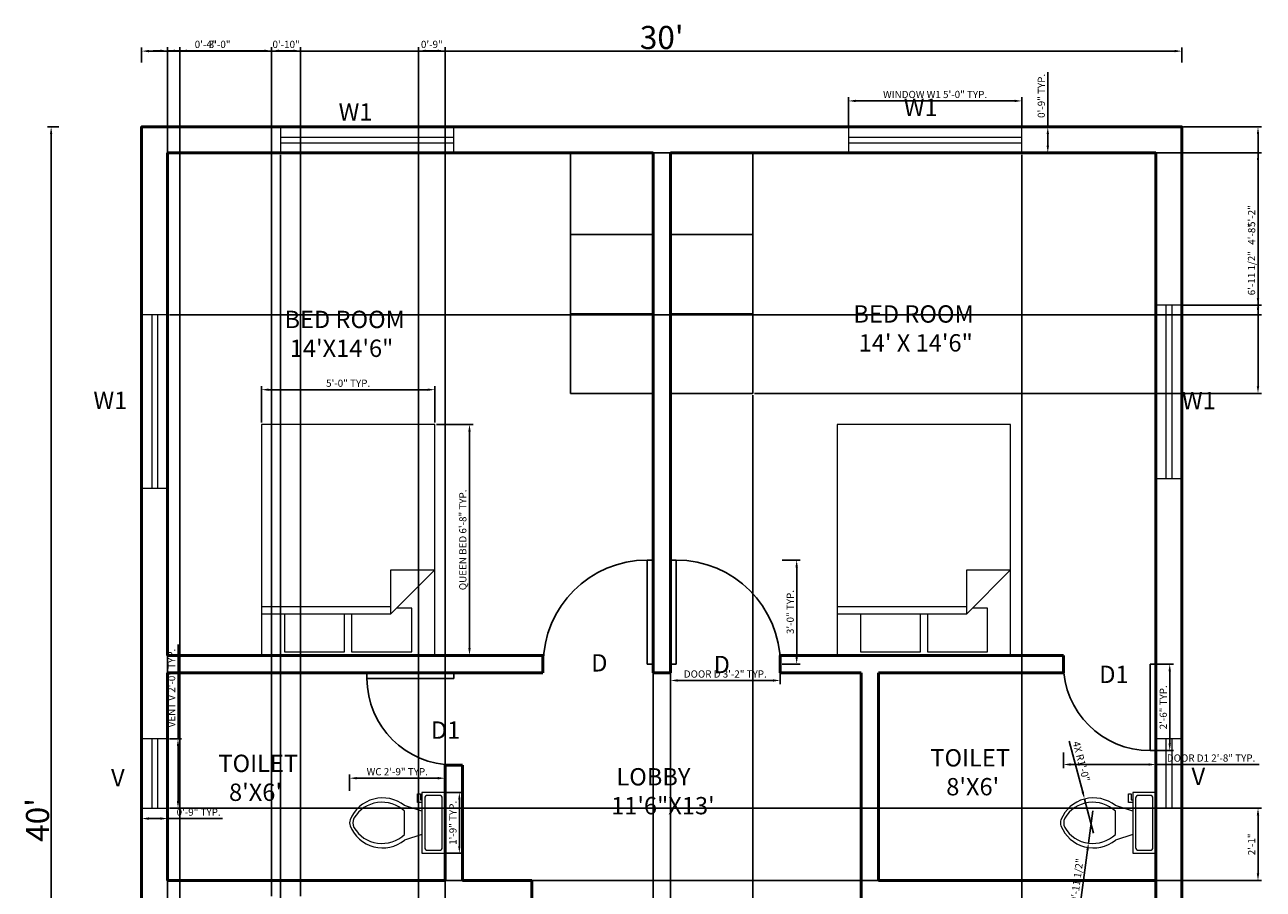
# Model space of a CAD drawing. Units: inches. Extents: x 2936 to 3364, y 2324 to 2867.
# Tile 4 of 4: x 2936 to 3364, y 2568 to 2867. Entities that reach past the tile are written whole.
import ezdxf

# ---------------------------------------------------------------- set-up
doc = ezdxf.new("R2010")
doc.units = ezdxf.units.IN
for name, color, linetype, lineweight in [('A-ANNO-DIMS', 2, 'Continuous', 18), ('A-ANNO-TEXT', 7, 'Continuous', 18), ('A-AREA-IDEN', 7, 'Continuous', 25), ('A-DOOR', 3, 'Continuous', 25), ('A-FLOR-CASE', 9, 'Continuous', 25), ('A-FLOR-FIXT', 9, 'Continuous', 18), ('A-FURN', 8, 'Continuous', 18), ('A-GLAZ', 4, 'Continuous', 18), ('A-WALL', 7, 'Continuous', 50)]:
    doc.layers.add(name, color=color, linetype=linetype, lineweight=lineweight)
doc.styles.get("Standard").update_dxf_attribs({"font": 'arial.ttf'})
doc.dimstyles.new('ISO-25', dxfattribs={"dimtxt": 2.5, "dimasz": 2.5, "dimexe": 1.25, "dimexo": 0.625, "dimtad": 1, "dimdec": 0, "dimlunit": 4, "dimtxsty": 'Standard', "dimcen": 2.5, "dimadec": 0, "dimazin": 0, "dimtfac": 1, "dimtdec": 0, "dimtmove": 0, "dimatfit": 3, "dimfxl": 1, "dimarcsym": 0})

# ---------------------------------------------------------------- blocks, each defined once
blk = doc.blocks.new('Toilet - top')
for p, q in [((9.5, -6), (9.5, -2)), ((-10, -8.5), (-8, -8.5)), ((-10, -9.5), (-10, -8.5)), ((-8, -8.5), (-8, -8)), ((-7, -8), (-7, -9.5)), ((-4, -8), (-6, -14)), ((4, -8), (6, -14)), ((-7, -9.5), (-10, -9.5)), ((4, -14), (-4, -14))]:
    blk.add_line(p, q)
blk.add_lwpolyline([(10.5, -8), (10.5, 0), (-10.5, 0), (-10.5, -8)], close=True)
for points in [[(-9.5, -2), (-9.5, -6)], [(8.5, -1), (-8.5, -1)], [(-8.5, -7), (8.5, -7)]]:
    blk.add_lwpolyline(points)
for centre, radius, start, end in [((-8.62, -1.88), 0.884, 81.8699, 188.1301), ((8.62, -1.88), 0.884, 351.8699, 98.1301), ((-8.62, -6.12), 0.884, 171.8699, 278.1301), ((8.62, -6.12), 0.884, 261.8699, 8.1301), ((3.52, -21.58), 12.17, 141.4691, 247.9714), ((4.2, -21.82), 11.33, 136.3677, 238.9468), ((-3.52, -21.58), 12.17, 292.0284, 38.5307), ((-4.2, -21.82), 11.33, 301.053, 43.6321), ((0, -27.88), 4, 245.7318, 294.2682), ((0, -29), 4, 254.8605, 285.1395)]:
    blk.add_arc(centre, radius, start, end)
blk = doc.blocks.new('Bed - Queen')
for p, q in [((0, -80.00003), (0, 0)), ((0, 0), (59.99999, 0)), ((59.99999, 0), (59.99999, -80.00003)), ((7.99999, -1.2), (28.79998, -1.2)), ((7.99999, -14.4), (7.99999, -1.2)), ((28.79998, -1.2), (28.79998, -14.4)), ((31.19999, -1.2), (51.99999, -1.2)), ((31.19999, -14.4), (31.19999, -1.2)), ((51.99999, -1.2), (51.99999, -16.4)), ((0, -14.4), (44.8, -14.4)), ((44.8, -16.8), (0, -16.8)), ((59.99999, -29.6), (44.8, -14.4)), ((44.8, -14.4), (44.8, -29.6)), ((51.99999, -16.4), (46.79936, -16.4)), ((44.8, -29.6), (59.99999, -29.6)), ((59.99999, -80.00003), (0, -80.00003))]:
    blk.add_line(p, q)
blk = doc.blocks.new('*D9')
at = {"layer": 'A-ANNO-DIMS', "color": 0, "lineweight": -2, "transparency": 16777216}
for p, q in [((2976.17, 2854.37), (2976.17, 2859.61)), ((3336.17, 2854.37), (3336.17, 2859.61)), ((2978.67, 2858.36), (3333.67, 2858.36))]:
    blk.add_line(p, q, dxfattribs=at)
at = {"layer": 'A-ANNO-DIMS', "color": 0, "transparency": 16777216}
for points in [[(2978.67, 2858.78), (2978.67, 2857.95), (2976.17, 2858.36)], [(3333.67, 2858.78), (3333.67, 2857.95), (3336.17, 2858.36)]]:
    blk.add_solid(points, dxfattribs=at)
at = {"layer": 'Defpoints', "color": 0, "transparency": 16777216}
for p in [(3336.17, 2858.36), (2976.17, 2853.74), (3336.17, 2853.74)]:
    blk.add_point(p, dxfattribs=at)
at = {"layer": 'A-ANNO-DIMS', "color": 0, "transparency": 16777216, "insert": (3156.17, 2863.08), "char_height": 2.5, "width": 17.9118, "attachment_point": 5}
blk.add_mtext("{\\H3.2x;30'}", dxfattribs=at)
blk = doc.blocks.new('*D10')
at = {"layer": 'A-ANNO-DIMS', "color": 0, "lineweight": -2, "transparency": 16777216}
for p, q in [((2947.52, 2832.11), (2943.61, 2832.11)), ((2944.86, 2829.61), (2944.86, 2354.61)), ((2947.52, 2352.11), (2943.61, 2352.11))]:
    blk.add_line(p, q, dxfattribs=at)
at = {"layer": 'A-ANNO-DIMS', "color": 0, "transparency": 16777216}
for points in [[(2944.44, 2829.61), (2945.27, 2829.61), (2944.86, 2832.11)], [(2944.44, 2354.61), (2945.27, 2354.61), (2944.86, 2352.11)]]:
    blk.add_solid(points, dxfattribs=at)
at = {"layer": 'Defpoints', "color": 0, "transparency": 16777216}
for p in [(2948.14, 2832.11), (2944.86, 2352.11), (2948.14, 2352.11)]:
    blk.add_point(p, dxfattribs=at)
at = {"layer": 'A-ANNO-DIMS', "color": 0, "transparency": 16777216, "insert": (2940.15, 2592.11), "char_height": 2.5, "width": 21.2299, "attachment_point": 5, "rotation": 90}
blk.add_mtext("{\\H3.2x;40'}", dxfattribs=at)
blk = doc.blocks.new('WIN-W1-60IN')
for p, q in [((3.5, 60), (3.5, 0)), ((5.5, 60), (5.5, 0))]:
    blk.add_line(p, q)
blk.add_lwpolyline([(0, 0), (9, 0), (9, 60), (0, 60)], close=True)
blk = doc.blocks.new('VENT-V-24IN')
for p, q in [((3.5, 24), (3.5, 0)), ((5.5, 24), (5.5, 0))]:
    blk.add_line(p, q)
blk.add_lwpolyline([(0, 0), (9, 0), (9, 24), (0, 24)], close=True)
blk = doc.blocks.new('DOOR-D1-30IN')
for p, q in [((0, -30), (0, 0)), ((0, 0), (2, 0)), ((2, 0), (2, -30)), ((2, -30), (0, -30))]:
    blk.add_line(p, q)
blk.add_arc((0, 0), 30, 180, 270)
blk = doc.blocks.new('DOOR-D-36IN')
for p, q in [((-2, 36), (0, 36)), ((0, 36), (0, 0)), ((-2, 0), (0, 0))]:
    blk.add_line(p, q)
blk.add_arc((0, 0), 36, 0, 90)
blk = doc.blocks.new('*D15')
at = {"layer": 'A-ANNO-DIMS', "color": 0, "lineweight": -2, "transparency": 16777216}
for p, q in [((3220.77, 2832.74), (3220.77, 2842.36)), ((3280.77, 2832.74), (3280.77, 2842.36)), ((3278.27, 2841.11), (3223.27, 2841.11))]:
    blk.add_line(p, q, dxfattribs=at)
at = {"layer": 'A-ANNO-DIMS', "color": 0, "transparency": 16777216}
for points in [[(3223.27, 2841.53), (3223.27, 2840.7), (3220.77, 2841.11)], [(3278.27, 2841.53), (3278.27, 2840.7), (3280.77, 2841.11)]]:
    blk.add_solid(points, dxfattribs=at)
at = {"layer": 'Defpoints', "color": 0, "transparency": 16777216}
for p in [(3220.77, 2841.11), (3220.77, 2832.11), (3280.77, 2832.11)]:
    blk.add_point(p, dxfattribs=at)
at = {"layer": 'A-ANNO-DIMS', "color": 0, "transparency": 16777216, "insert": (3250.77, 2843.03), "char_height": 2.5, "attachment_point": 5}
blk.add_mtext('WINDOW W1 5\'-0" TYP.', dxfattribs=at)
blk = doc.blocks.new('*D16')
at = {"layer": 'A-ANNO-DIMS', "color": 0, "lineweight": -2, "transparency": 16777216}
for p, q in [((3289.77, 2832.11), (3289.77, 2851.1)), ((3281.4, 2832.11), (3291.02, 2832.11)), ((3289.77, 2825.61), (3289.77, 2829.61)), ((3281.4, 2823.11), (3291.02, 2823.11))]:
    blk.add_line(p, q, dxfattribs=at)
at = {"layer": 'A-ANNO-DIMS', "color": 0, "transparency": 16777216}
for points in [[(3289.36, 2829.61), (3290.19, 2829.61), (3289.77, 2832.11)], [(3289.36, 2825.61), (3290.19, 2825.61), (3289.77, 2823.11)]]:
    blk.add_solid(points, dxfattribs=at)
at = {"layer": 'Defpoints', "color": 0, "transparency": 16777216}
for p in [(3280.77, 2832.11), (3289.77, 2832.11), (3280.77, 2823.11)]:
    blk.add_point(p, dxfattribs=at)
at = {"layer": 'A-ANNO-DIMS', "color": 0, "transparency": 16777216, "insert": (3287.87, 2842.86), "char_height": 2.5, "attachment_point": 5, "rotation": 90}
blk.add_mtext('0\'-9" TYP.', dxfattribs=at)
blk = doc.blocks.new('*D17')
at = {"layer": 'A-ANNO-DIMS', "color": 0, "lineweight": -2, "transparency": 16777216}
for p, q in [((2988.77, 2620.19), (2988.77, 2652.89)), ((2985.79, 2620.19), (2990.02, 2620.19)), ((2988.77, 2598.69), (2988.77, 2617.69)), ((2985.79, 2596.19), (2990.02, 2596.19))]:
    blk.add_line(p, q, dxfattribs=at)
at = {"layer": 'A-ANNO-DIMS', "color": 0, "transparency": 16777216}
for points in [[(2988.35, 2617.69), (2989.19, 2617.69), (2988.77, 2620.19)], [(2988.35, 2598.69), (2989.19, 2598.69), (2988.77, 2596.19)]]:
    blk.add_solid(points, dxfattribs=at)
at = {"layer": 'Defpoints', "color": 0, "transparency": 16777216}
for p in [(2985.17, 2620.19), (2988.77, 2620.19), (2985.17, 2596.19)]:
    blk.add_point(p, dxfattribs=at)
at = {"layer": 'A-ANNO-DIMS', "color": 0, "transparency": 16777216, "insert": (2986.87, 2637.79), "char_height": 2.5, "attachment_point": 5, "rotation": 90}
blk.add_mtext('VENT V 2\'-0" TYP.', dxfattribs=at)
blk = doc.blocks.new('*D18')
at = {"layer": 'A-ANNO-DIMS', "color": 0, "lineweight": -2, "transparency": 16777216}
for p, q in [((2976.17, 2595.57), (2976.17, 2591.34)), ((2985.17, 2595.57), (2985.17, 2591.34)), ((2978.67, 2592.59), (2982.67, 2592.59)), ((2985.17, 2592.59), (3004.16, 2592.59))]:
    blk.add_line(p, q, dxfattribs=at)
at = {"layer": 'A-ANNO-DIMS', "color": 0, "transparency": 16777216}
for points in [[(2978.67, 2593.01), (2978.67, 2592.17), (2976.17, 2592.59)], [(2982.67, 2593.01), (2982.67, 2592.17), (2985.17, 2592.59)]]:
    blk.add_solid(points, dxfattribs=at)
at = {"layer": 'Defpoints', "color": 0, "transparency": 16777216}
for p in [(2976.17, 2596.19), (2985.17, 2596.19), (2985.17, 2592.59)]:
    blk.add_point(p, dxfattribs=at)
at = {"layer": 'A-ANNO-DIMS', "color": 0, "transparency": 16777216, "insert": (2995.91, 2594.49), "char_height": 2.5, "attachment_point": 5}
blk.add_mtext('0\'-9" TYP.', dxfattribs=at)
blk = doc.blocks.new('*D19')
at = {"layer": 'A-ANNO-DIMS', "color": 0, "lineweight": -2, "transparency": 16777216}
for p, q in [((3159.17, 2645.49), (3159.17, 2639.16)), ((3197.17, 2645.49), (3197.17, 2639.16)), ((3161.67, 2640.41), (3194.67, 2640.41))]:
    blk.add_line(p, q, dxfattribs=at)
at = {"layer": 'A-ANNO-DIMS', "color": 0, "transparency": 16777216}
for points in [[(3161.67, 2640.83), (3161.67, 2640), (3159.17, 2640.41)], [(3194.67, 2640.83), (3194.67, 2640), (3197.17, 2640.41)]]:
    blk.add_solid(points, dxfattribs=at)
at = {"layer": 'Defpoints', "color": 0, "transparency": 16777216}
for p in [(3159.17, 2646.11), (3197.17, 2646.11), (3197.17, 2640.41)]:
    blk.add_point(p, dxfattribs=at)
at = {"layer": 'A-ANNO-DIMS', "color": 0, "transparency": 16777216, "insert": (3178.17, 2642.33), "char_height": 2.5, "attachment_point": 5}
blk.add_mtext('DOOR D 3\'-2" TYP.', dxfattribs=at)
blk = doc.blocks.new('*D20')
at = {"layer": 'A-ANNO-DIMS', "color": 0, "lineweight": -2, "transparency": 16777216}
for p, q in [((3197.79, 2682.11), (3204.12, 2682.11)), ((3202.87, 2648.61), (3202.87, 2679.61)), ((3197.79, 2646.11), (3204.12, 2646.11))]:
    blk.add_line(p, q, dxfattribs=at)
at = {"layer": 'A-ANNO-DIMS', "color": 0, "transparency": 16777216}
for points in [[(3202.45, 2679.61), (3203.29, 2679.61), (3202.87, 2682.11)], [(3202.45, 2648.61), (3203.29, 2648.61), (3202.87, 2646.11)]]:
    blk.add_solid(points, dxfattribs=at)
at = {"layer": 'Defpoints', "color": 0, "transparency": 16777216}
for p in [(3197.17, 2682.11), (3202.87, 2682.11), (3197.17, 2646.11)]:
    blk.add_point(p, dxfattribs=at)
at = {"layer": 'A-ANNO-DIMS', "color": 0, "transparency": 16777216, "insert": (3200.97, 2664.11), "char_height": 2.5, "attachment_point": 5, "rotation": 90}
blk.add_mtext('3\'-0" TYP.', dxfattribs=at)
blk = doc.blocks.new('*D21')
at = {"layer": 'A-ANNO-DIMS', "color": 0, "lineweight": -2, "transparency": 16777216}
for p, q in [((3295.17, 2615.49), (3295.17, 2610.06)), ((3327.17, 2615.49), (3327.17, 2610.06)), ((3297.67, 2611.31), (3324.67, 2611.31)), ((3327.17, 2611.31), (3362.92, 2611.31))]:
    blk.add_line(p, q, dxfattribs=at)
at = {"layer": 'A-ANNO-DIMS', "color": 0, "transparency": 16777216}
for points in [[(3297.67, 2611.73), (3297.67, 2610.9), (3295.17, 2611.31)], [(3324.67, 2611.73), (3324.67, 2610.9), (3327.17, 2611.31)]]:
    blk.add_solid(points, dxfattribs=at)
at = {"layer": 'Defpoints', "color": 0, "transparency": 16777216}
for p in [(3295.17, 2616.11), (3327.17, 2616.11), (3327.17, 2611.31)]:
    blk.add_point(p, dxfattribs=at)
at = {"layer": 'A-ANNO-DIMS', "color": 0, "transparency": 16777216, "insert": (3346.29, 2613.23), "char_height": 2.5, "attachment_point": 5}
blk.add_mtext('DOOR D1 2\'-8" TYP.', dxfattribs=at)
blk = doc.blocks.new('*D22')
at = {"layer": 'A-ANNO-DIMS', "color": 0, "lineweight": -2, "transparency": 16777216}
for p, q in [((3327.79, 2646.11), (3333.22, 2646.11)), ((3331.97, 2618.61), (3331.97, 2643.61)), ((3327.79, 2616.11), (3333.22, 2616.11))]:
    blk.add_line(p, q, dxfattribs=at)
at = {"layer": 'A-ANNO-DIMS', "color": 0, "transparency": 16777216}
for points in [[(3331.55, 2643.61), (3332.39, 2643.61), (3331.97, 2646.11)], [(3331.55, 2618.61), (3332.39, 2618.61), (3331.97, 2616.11)]]:
    blk.add_solid(points, dxfattribs=at)
at = {"layer": 'Defpoints', "color": 0, "transparency": 16777216}
for p in [(3327.17, 2646.11), (3331.97, 2646.11), (3327.17, 2616.11)]:
    blk.add_point(p, dxfattribs=at)
at = {"layer": 'A-ANNO-DIMS', "color": 0, "transparency": 16777216, "insert": (3330.07, 2631.11), "char_height": 2.5, "attachment_point": 5, "rotation": 90}
blk.add_mtext('2\'-6" TYP.', dxfattribs=at)
blk = doc.blocks.new('*D23')
at = {"layer": 'A-ANNO-DIMS', "color": 0, "lineweight": -2, "transparency": 16777216}
for p, q in [((3078.27, 2729.11), (3090.89, 2729.11)), ((3089.64, 2726.61), (3089.64, 2651.61)), ((3078.27, 2649.11), (3090.89, 2649.11))]:
    blk.add_line(p, q, dxfattribs=at)
at = {"layer": 'A-ANNO-DIMS', "color": 0, "transparency": 16777216}
for points in [[(3089.23, 2726.61), (3090.06, 2726.61), (3089.64, 2729.11)], [(3089.23, 2651.61), (3090.06, 2651.61), (3089.64, 2649.11)]]:
    blk.add_solid(points, dxfattribs=at)
at = {"layer": 'Defpoints', "color": 0, "transparency": 16777216}
for p in [(3077.64, 2729.11), (3077.64, 2649.11), (3089.64, 2649.11)]:
    blk.add_point(p, dxfattribs=at)
at = {"layer": 'A-ANNO-DIMS', "color": 0, "transparency": 16777216, "insert": (3087.65, 2689.11), "char_height": 2.5, "attachment_point": 5, "rotation": 90}
blk.add_mtext('QUEEN BED 6\'-8" TYP.', dxfattribs=at)
blk = doc.blocks.new('*D24')
at = {"layer": 'A-ANNO-DIMS', "color": 0, "lineweight": -2, "transparency": 16777216}
for p, q in [((3017.64, 2729.74), (3017.64, 2742.36)), ((3020.14, 2741.11), (3075.14, 2741.11)), ((3077.64, 2729.74), (3077.64, 2742.36))]:
    blk.add_line(p, q, dxfattribs=at)
at = {"layer": 'A-ANNO-DIMS', "color": 0, "transparency": 16777216}
for points in [[(3020.14, 2741.53), (3020.14, 2740.7), (3017.64, 2741.11)], [(3075.14, 2741.53), (3075.14, 2740.7), (3077.64, 2741.11)]]:
    blk.add_solid(points, dxfattribs=at)
at = {"layer": 'Defpoints', "color": 0, "transparency": 16777216}
for p in [(3077.64, 2741.11), (3017.64, 2729.11), (3077.64, 2729.11)]:
    blk.add_point(p, dxfattribs=at)
at = {"layer": 'A-ANNO-DIMS', "color": 0, "transparency": 16777216, "insert": (3047.64, 2743.02), "char_height": 2.5, "attachment_point": 5}
blk.add_mtext('5\'-0" TYP.', dxfattribs=at)
blk = doc.blocks.new('*D25')
at = {"layer": 'A-ANNO-DIMS', "color": 0, "lineweight": -2, "transparency": 16777216}
for p, q in [((3048.12, 2602.24), (3048.12, 2607.82)), ((3050.62, 2606.57), (3078.67, 2606.57)), ((3081.17, 2602.24), (3081.17, 2607.82))]:
    blk.add_line(p, q, dxfattribs=at)
at = {"layer": 'A-ANNO-DIMS', "color": 0, "transparency": 16777216}
for points in [[(3050.62, 2606.99), (3050.62, 2606.15), (3048.12, 2606.57)], [(3078.67, 2606.99), (3078.67, 2606.15), (3081.17, 2606.57)]]:
    blk.add_solid(points, dxfattribs=at)
at = {"layer": 'Defpoints', "color": 0, "transparency": 16777216}
for p in [(3081.17, 2606.57), (3048.12, 2601.61), (3081.17, 2601.61)]:
    blk.add_point(p, dxfattribs=at)
at = {"layer": 'A-ANNO-DIMS', "color": 0, "transparency": 16777216, "insert": (3064.65, 2608.49), "char_height": 2.5, "attachment_point": 5}
blk.add_mtext('WC 2\'-9" TYP.', dxfattribs=at)
blk = doc.blocks.new('*D26')
at = {"layer": 'A-ANNO-DIMS', "color": 0, "lineweight": -2, "transparency": 16777216}
for p, q in [((3081.79, 2601.61), (3087.38, 2601.61)), ((3086.13, 2599.11), (3086.13, 2583.11)), ((3081.79, 2580.61), (3087.38, 2580.61))]:
    blk.add_line(p, q, dxfattribs=at)
at = {"layer": 'A-ANNO-DIMS', "color": 0, "transparency": 16777216}
for points in [[(3085.71, 2599.11), (3086.54, 2599.11), (3086.13, 2601.61)], [(3085.71, 2583.11), (3086.54, 2583.11), (3086.13, 2580.61)]]:
    blk.add_solid(points, dxfattribs=at)
at = {"layer": 'Defpoints', "color": 0, "transparency": 16777216}
for p in [(3081.17, 2601.61), (3081.17, 2580.61), (3086.13, 2580.61)]:
    blk.add_point(p, dxfattribs=at)
at = {"layer": 'A-ANNO-DIMS', "color": 0, "transparency": 16777216, "insert": (3084.23, 2591.11), "char_height": 2.5, "attachment_point": 5, "rotation": 90}
blk.add_mtext('1\'-9" TYP.', dxfattribs=at)
blk = doc.blocks.new('*D40')
at = {"layer": 'A-ANNO-DIMS', "color": 0, "lineweight": -2, "transparency": 16777216}
for p, q in [((2985.79, 2823.11), (3363.77, 2823.11)), ((3362.52, 2820.61), (3362.52, 2769.5)), ((2985.79, 2767), (3363.77, 2767))]:
    blk.add_line(p, q, dxfattribs=at)
at = {"layer": 'A-ANNO-DIMS', "color": 0, "transparency": 16777216}
for points in [[(3362.1, 2820.61), (3362.94, 2820.61), (3362.52, 2823.11)], [(3362.1, 2769.5), (3362.94, 2769.5), (3362.52, 2767)]]:
    blk.add_solid(points, dxfattribs=at)
at = {"layer": 'Defpoints', "color": 0, "transparency": 16777216}
for p in [(2985.17, 2823.11), (2985.17, 2767), (3362.52, 2767)]:
    blk.add_point(p, dxfattribs=at)
at = {"layer": 'A-ANNO-DIMS', "color": 0, "transparency": 16777216, "insert": (3360.62, 2795.06), "char_height": 2.5, "attachment_point": 5, "rotation": 90}
blk.add_mtext('4\'-8"', dxfattribs=at)
blk = doc.blocks.new('*D41')
at = {"layer": 'A-ANNO-DIMS', "color": 0, "lineweight": -2, "transparency": 16777216}
for p, q in [((3336.79, 2832.11), (3363.77, 2832.11)), ((3362.52, 2829.61), (3362.52, 2772.85)), ((3336.79, 2770.35), (3363.77, 2770.35))]:
    blk.add_line(p, q, dxfattribs=at)
at = {"layer": 'A-ANNO-DIMS', "color": 0, "transparency": 16777216}
for points in [[(3362.1, 2829.61), (3362.94, 2829.61), (3362.52, 2832.11)], [(3362.1, 2772.85), (3362.94, 2772.85), (3362.52, 2770.35)]]:
    blk.add_solid(points, dxfattribs=at)
at = {"layer": 'Defpoints', "color": 0, "transparency": 16777216}
for p in [(3336.17, 2832.11), (3336.17, 2770.35), (3362.52, 2770.35)]:
    blk.add_point(p, dxfattribs=at)
at = {"layer": 'A-ANNO-DIMS', "color": 0, "transparency": 16777216, "insert": (3360.62, 2801.23), "char_height": 2.5, "attachment_point": 5, "rotation": 90}
blk.add_mtext('5\'-2"', dxfattribs=at)
blk = doc.blocks.new('*D43')
at = {"layer": 'A-ANNO-DIMS', "color": 0, "lineweight": -2, "transparency": 16777216}
for p, q in [((2985.17, 2822.49), (2985.17, 2324.51)), ((3024.27, 2822.49), (3024.27, 2324.51)), ((2987.67, 2325.76), (3021.77, 2325.76))]:
    blk.add_line(p, q, dxfattribs=at)
at = {"layer": 'A-ANNO-DIMS', "color": 0, "transparency": 16777216}
for points in [[(2987.67, 2326.18), (2987.67, 2325.35), (2985.17, 2325.76)], [(3021.77, 2326.18), (3021.77, 2325.35), (3024.27, 2325.76)]]:
    blk.add_solid(points, dxfattribs=at)
at = {"layer": 'Defpoints', "color": 0, "transparency": 16777216}
for p in [(2985.17, 2823.11), (3024.27, 2823.11), (3024.27, 2325.76)]:
    blk.add_point(p, dxfattribs=at)
at = {"layer": 'A-ANNO-DIMS', "color": 0, "transparency": 16777216, "insert": (3004.72, 2327.67), "char_height": 2.5, "attachment_point": 5}
blk.add_mtext('3\'-3"', dxfattribs=at)
blk = doc.blocks.new('*D44')
at = {"layer": 'A-ANNO-DIMS', "color": 0, "lineweight": -2, "transparency": 16777216}
for p, q in [((3280.77, 2822.49), (3280.77, 2324.51)), ((3327.17, 2822.49), (3327.17, 2324.51)), ((3283.27, 2325.76), (3324.67, 2325.76))]:
    blk.add_line(p, q, dxfattribs=at)
at = {"layer": 'A-ANNO-DIMS', "color": 0, "transparency": 16777216}
for points in [[(3283.27, 2326.18), (3283.27, 2325.35), (3280.77, 2325.76)], [(3324.67, 2326.18), (3324.67, 2325.35), (3327.17, 2325.76)]]:
    blk.add_solid(points, dxfattribs=at)
at = {"layer": 'Defpoints', "color": 0, "transparency": 16777216}
for p in [(3280.77, 2823.11), (3327.17, 2823.11), (3327.17, 2325.76)]:
    blk.add_point(p, dxfattribs=at)
at = {"layer": 'A-ANNO-DIMS', "color": 0, "transparency": 16777216, "insert": (3303.97, 2327.68), "char_height": 2.5, "attachment_point": 5}
blk.add_mtext('3\'-10 1/2"', dxfattribs=at)
blk = doc.blocks.new('*D47')
at = {"layer": 'A-ANNO-DIMS', "color": 0, "lineweight": -2, "transparency": 16777216}
for p, q in [((3327.79, 2596.19), (3363.77, 2596.19)), ((3362.52, 2573.61), (3362.52, 2593.69)), ((3327.79, 2571.11), (3363.77, 2571.11))]:
    blk.add_line(p, q, dxfattribs=at)
at = {"layer": 'A-ANNO-DIMS', "color": 0, "transparency": 16777216}
for points in [[(3362.1, 2593.69), (3362.94, 2593.69), (3362.52, 2596.19)], [(3362.1, 2573.61), (3362.94, 2573.61), (3362.52, 2571.11)]]:
    blk.add_solid(points, dxfattribs=at)
at = {"layer": 'Defpoints', "color": 0, "transparency": 16777216}
for p in [(3327.17, 2596.19), (3362.52, 2596.19), (3327.17, 2571.11)]:
    blk.add_point(p, dxfattribs=at)
at = {"layer": 'A-ANNO-DIMS', "color": 0, "transparency": 16777216, "insert": (3360.64, 2583.65), "char_height": 2.5, "attachment_point": 5, "rotation": 90}
blk.add_mtext('2\'-1"', dxfattribs=at)
blk = doc.blocks.new('*D48')
at = {"layer": 'A-ANNO-DIMS', "color": 0, "lineweight": -2, "transparency": 16777216}
for p, q in [((2985.17, 2565.74), (2985.17, 2859.71)), ((3021.17, 2565.74), (3021.17, 2859.71)), ((2987.67, 2858.46), (3018.67, 2858.46))]:
    blk.add_line(p, q, dxfattribs=at)
at = {"layer": 'A-ANNO-DIMS', "color": 0, "transparency": 16777216}
for points in [[(2987.67, 2858.88), (2987.67, 2858.05), (2985.17, 2858.46)], [(3018.67, 2858.88), (3018.67, 2858.05), (3021.17, 2858.46)]]:
    blk.add_solid(points, dxfattribs=at)
at = {"layer": 'Defpoints', "color": 0, "transparency": 16777216}
for p in [(3021.17, 2858.46), (2985.17, 2565.11), (3021.17, 2565.11)]:
    blk.add_point(p, dxfattribs=at)
at = {"layer": 'A-ANNO-DIMS', "color": 0, "transparency": 16777216, "insert": (3003.17, 2860.37), "char_height": 2.5, "attachment_point": 5}
blk.add_mtext('3\'-0"', dxfattribs=at)
blk = doc.blocks.new('*D49')
at = {"layer": 'A-ANNO-DIMS', "color": 0, "lineweight": -2, "transparency": 16777216}
for p, q in [((3021.17, 2565.74), (3021.17, 2859.71)), ((3031.17, 2565.74), (3031.17, 2859.71)), ((3023.67, 2858.46), (3028.67, 2858.46))]:
    blk.add_line(p, q, dxfattribs=at)
at = {"layer": 'A-ANNO-DIMS', "color": 0, "transparency": 16777216}
for points in [[(3023.67, 2858.88), (3023.67, 2858.05), (3021.17, 2858.46)], [(3028.67, 2858.88), (3028.67, 2858.05), (3031.17, 2858.46)]]:
    blk.add_solid(points, dxfattribs=at)
at = {"layer": 'Defpoints', "color": 0, "transparency": 16777216}
for p in [(3031.17, 2858.46), (3021.17, 2565.11), (3031.17, 2565.11)]:
    blk.add_point(p, dxfattribs=at)
at = {"layer": 'A-ANNO-DIMS', "color": 0, "transparency": 16777216, "insert": (3026.17, 2860.37), "char_height": 2.5, "attachment_point": 5}
blk.add_mtext('0\'-10"', dxfattribs=at)
blk = doc.blocks.new('*D51')
at = {"layer": 'A-ANNO-DIMS', "color": 0, "lineweight": -2, "transparency": 16777216}
for p, q in [((3153.17, 2822.49), (3153.17, 2324.51)), ((3159.17, 2822.49), (3159.17, 2324.51)), ((3150.67, 2325.76), (3148.17, 2325.76)), ((3153.17, 2325.76), (3159.17, 2325.76)), ((3161.67, 2325.76), (3172.07, 2325.76))]:
    blk.add_line(p, q, dxfattribs=at)
at = {"layer": 'A-ANNO-DIMS', "color": 0, "transparency": 16777216}
for points in [[(3150.67, 2326.18), (3150.67, 2325.35), (3153.17, 2325.76)], [(3161.67, 2326.18), (3161.67, 2325.35), (3159.17, 2325.76)]]:
    blk.add_solid(points, dxfattribs=at)
at = {"layer": 'Defpoints', "color": 0, "transparency": 16777216}
for p in [(3153.17, 2823.11), (3159.17, 2823.11), (3159.17, 2325.76)]:
    blk.add_point(p, dxfattribs=at)
at = {"layer": 'A-ANNO-DIMS', "color": 0, "transparency": 16777216, "insert": (3168.12, 2327.67), "char_height": 2.5, "attachment_point": 5}
blk.add_mtext('0\'-6"', dxfattribs=at)
blk = doc.blocks.new('*D52')
at = {"layer": 'A-ANNO-DIMS', "color": 0, "lineweight": -2, "transparency": 16777216}
for p, q in [((3188.33, 2823.11), (3363.77, 2823.11)), ((3362.52, 2820.61), (3362.52, 2742.31)), ((3188.33, 2739.81), (3363.77, 2739.81))]:
    blk.add_line(p, q, dxfattribs=at)
at = {"layer": 'A-ANNO-DIMS', "color": 0, "transparency": 16777216}
for points in [[(3362.1, 2820.61), (3362.94, 2820.61), (3362.52, 2823.11)], [(3362.1, 2742.31), (3362.94, 2742.31), (3362.52, 2739.81)]]:
    blk.add_solid(points, dxfattribs=at)
at = {"layer": 'Defpoints', "color": 0, "transparency": 16777216}
for p in [(3187.71, 2823.11), (3187.71, 2739.81), (3362.52, 2739.81)]:
    blk.add_point(p, dxfattribs=at)
at = {"layer": 'A-ANNO-DIMS', "color": 0, "transparency": 16777216, "insert": (3360.6, 2781.46), "char_height": 2.5, "attachment_point": 5, "rotation": 90}
blk.add_mtext('6\'-11 1/2"', dxfattribs=at)
blk = doc.blocks.new('*D53')
at = {"layer": 'A-ANNO-DIMS', "color": 0, "lineweight": -2, "transparency": 16777216}
for p, q in [((3159.17, 2739.18), (3159.17, 2324.51)), ((3187.71, 2739.18), (3187.71, 2324.51)), ((3161.67, 2325.76), (3185.21, 2325.76))]:
    blk.add_line(p, q, dxfattribs=at)
at = {"layer": 'A-ANNO-DIMS', "color": 0, "transparency": 16777216}
for points in [[(3161.67, 2326.18), (3161.67, 2325.35), (3159.17, 2325.76)], [(3185.21, 2326.18), (3185.21, 2325.35), (3187.71, 2325.76)]]:
    blk.add_solid(points, dxfattribs=at)
at = {"layer": 'Defpoints', "color": 0, "transparency": 16777216}
for p in [(3159.17, 2739.81), (3187.71, 2739.81), (3187.71, 2325.76)]:
    blk.add_point(p, dxfattribs=at)
at = {"layer": 'A-ANNO-DIMS', "color": 0, "transparency": 16777216, "insert": (3173.44, 2327.68), "char_height": 2.5, "attachment_point": 5}
blk.add_mtext('2\'-4 1/2"', dxfattribs=at)
blk = doc.blocks.new('*D57')
at = {"layer": 'A-ANNO-DIMS', "color": 0, "lineweight": -2, "transparency": 16777216}
for p, q in [((2985.79, 2596.19), (3363.77, 2596.19)), ((3362.52, 2573.61), (3362.52, 2593.69)), ((2985.79, 2571.11), (3363.77, 2571.11))]:
    blk.add_line(p, q, dxfattribs=at)
at = {"layer": 'A-ANNO-DIMS', "color": 0, "transparency": 16777216}
for points in [[(3362.1, 2593.69), (3362.94, 2593.69), (3362.52, 2596.19)], [(3362.1, 2573.61), (3362.94, 2573.61), (3362.52, 2571.11)]]:
    blk.add_solid(points, dxfattribs=at)
at = {"layer": 'Defpoints', "color": 0, "transparency": 16777216}
for p in [(2985.17, 2596.19), (3362.52, 2596.19), (2985.17, 2571.11)]:
    blk.add_point(p, dxfattribs=at)
at = {"layer": 'A-ANNO-DIMS', "color": 0, "transparency": 16777216, "insert": (3360.64, 2583.65), "char_height": 2.5, "attachment_point": 5, "rotation": 90}
blk.add_mtext('2\'-1"', dxfattribs=at)
blk = doc.blocks.new('*D61')
at = {"layer": 'A-ANNO-DIMS', "color": 0, "lineweight": -2, "transparency": 16777216}
for p, q in [((2985.17, 2391.74), (2985.17, 2859.71)), ((2989.36, 2384.98), (2989.36, 2859.71)), ((2982.67, 2858.46), (2980.17, 2858.46)), ((2985.17, 2858.46), (2989.36, 2858.46)), ((2991.86, 2858.46), (3002.26, 2858.46))]:
    blk.add_line(p, q, dxfattribs=at)
at = {"layer": 'A-ANNO-DIMS', "color": 0, "transparency": 16777216}
for points in [[(2982.67, 2858.88), (2982.67, 2858.05), (2985.17, 2858.46)], [(2991.86, 2858.88), (2991.86, 2858.05), (2989.36, 2858.46)]]:
    blk.add_solid(points, dxfattribs=at)
at = {"layer": 'Defpoints', "color": 0, "transparency": 16777216}
for p in [(2989.36, 2858.46), (2985.17, 2391.11), (2989.36, 2384.35)]:
    blk.add_point(p, dxfattribs=at)
at = {"layer": 'A-ANNO-DIMS', "color": 0, "transparency": 16777216, "insert": (2998.31, 2860.37), "char_height": 2.5, "attachment_point": 5}
blk.add_mtext('0\'-4"', dxfattribs=at)
blk = doc.blocks.new('*D62')
at = {"layer": 'A-ANNO-DIMS', "color": 0, "lineweight": -2, "transparency": 16777216}
for p, q in [((3072.03, 2387.74), (3072.03, 2859.71)), ((3081.17, 2391.74), (3081.17, 2859.71)), ((3078.67, 2858.46), (3074.53, 2858.46))]:
    blk.add_line(p, q, dxfattribs=at)
at = {"layer": 'A-ANNO-DIMS', "color": 0, "transparency": 16777216}
for points in [[(3074.53, 2858.88), (3074.53, 2858.05), (3072.03, 2858.46)], [(3078.67, 2858.88), (3078.67, 2858.05), (3081.17, 2858.46)]]:
    blk.add_solid(points, dxfattribs=at)
at = {"layer": 'Defpoints', "color": 0, "transparency": 16777216}
for p in [(3072.03, 2858.46), (3081.17, 2391.11), (3072.03, 2387.11)]:
    blk.add_point(p, dxfattribs=at)
at = {"layer": 'A-ANNO-DIMS', "color": 0, "transparency": 16777216, "insert": (3076.6, 2860.37), "char_height": 2.5, "attachment_point": 5}
blk.add_mtext('0\'-9"', dxfattribs=at)
blk = doc.blocks.new('*D65')
at = {"layer": 'A-ANNO-DIMS', "color": 0, "lineweight": -2, "transparency": 16777216}
for p, q in [((3297.22, 2619.44), (3301.86, 2601.78)), ((3305.59, 2587.59), (3302.5, 2599.36))]:
    blk.add_line(p, q, dxfattribs=at)
at = {"layer": 'A-ANNO-DIMS', "color": 0, "transparency": 16777216}
blk.add_solid([(3302.26, 2601.89), (3301.46, 2601.68), (3302.5, 2599.36)], dxfattribs=at)
at = {"layer": 'Defpoints', "color": 0, "transparency": 16777216}
for p in [(3302.5, 2599.36), (3305.59, 2587.59)]:
    blk.add_point(p, dxfattribs=at)
at = {"layer": 'A-ANNO-DIMS', "color": 0, "transparency": 16777216, "insert": (3301.06, 2612.3), "char_height": 2.5, "attachment_point": 5, "rotation": 284.7207}
blk.add_mtext('4X R1\'-0"', dxfattribs=at)
blk = doc.blocks.new('*D66')
at = {"layer": 'A-ANNO-DIMS', "color": 0, "lineweight": -2, "transparency": 16777216}
for p, q in [((3305.35, 2595.31), (3303.84, 2584.09)), ((3300.04, 2555.81), (3303.51, 2581.61))]:
    blk.add_line(p, q, dxfattribs=at)
at = {"layer": 'A-ANNO-DIMS', "color": 0, "transparency": 16777216}
blk.add_solid([(3303.1, 2581.66), (3303.92, 2581.55), (3303.84, 2584.09)], dxfattribs=at)
at = {"layer": 'Defpoints', "color": 0, "transparency": 16777216}
for p in [(3305.35, 2595.31), (3303.84, 2584.09)]:
    blk.add_point(p, dxfattribs=at)
at = {"layer": 'A-ANNO-DIMS', "color": 0, "transparency": 16777216, "insert": (3299.71, 2567.73), "char_height": 2.5, "attachment_point": 5, "rotation": 82.3437}
blk.add_mtext('4X R0\'-11 1/2"', dxfattribs=at)

msp = doc.modelspace()

# ---------------------------------------------------------------- linework, layer by layer
at = {"layer": 'A-DOOR'}
for p, q in [((3159.17, 2646.11), (3159.17, 2682.11)), ((3197.17, 2646.11), (3197.17, 2649.11)), ((3084.17, 2611.11), (3087.17, 2611.11))]:
    msp.add_line(p, q, dxfattribs=at)
at = {"layer": 'A-FLOR-CASE'}
for p, q in [((3124.63, 2823.11), (3124.63, 2739.81)), ((3187.71, 2823.11), (3187.71, 2739.81)), ((3124.63, 2794.9), (3153.17, 2794.9)), ((3187.71, 2794.9), (3159.17, 2794.9)), ((3124.63, 2767.35), (3153.17, 2767.35)), ((3187.71, 2767.35), (3159.17, 2767.35))]:
    msp.add_line(p, q, dxfattribs=at)
for points in [[(3124.63, 2739.81), (3153.17, 2739.81), (3153.17, 2823.11), (3124.63, 2823.11)], [(3187.71, 2739.81), (3159.17, 2739.81), (3159.17, 2823.11), (3195.02, 2823.11)]]:
    msp.add_lwpolyline(points, dxfattribs=at)
at = {"layer": 'A-WALL'}
for p, q in [((2985.17, 2823.11), (2985.17, 2649.11)), ((3153.17, 2823.11), (2985.17, 2823.11)), ((3153.17, 2823.11), (3153.17, 2649.11)), ((3327.17, 2823.11), (3159.17, 2823.11)), ((3159.17, 2649.11), (3159.17, 2823.11)), ((3327.17, 2649.11), (3327.17, 2823.11)), ((3115.29, 2649.11), (2985.17, 2649.11)), ((3115.07, 2649.11), (3115.07, 2643.11)), ((3153.17, 2649.11), (3153.17, 2643.11)), ((3159.17, 2649.11), (3159.17, 2643.11)), ((3295.17, 2649.11), (3197.17, 2649.11)), ((3197.17, 2649.11), (3197.17, 2643.11)), ((3295.17, 2649.11), (3295.17, 2643.11)), ((3327.17, 2649.11), (3327.17, 2643.11)), ((2985.17, 2643.11), (2985.17, 2571.11)), ((3081.17, 2643.11), (2985.17, 2643.11)), ((3087.17, 2643.11), (3081.17, 2643.11)), ((3115.07, 2643.11), (3087.17, 2643.11)), ((3159.17, 2643.11), (3153.17, 2643.11)), ((3225.17, 2643.11), (3197.17, 2643.11)), ((3225.17, 2565.11), (3225.17, 2643.11)), ((3295.17, 2643.11), (3231.17, 2643.11)), ((3231.17, 2571.11), (3231.17, 2643.11)), ((3327.17, 2487.11), (3327.17, 2643.11)), ((3081.17, 2611.11), (3081.17, 2571.11)), ((3087.17, 2611.11), (3081.17, 2611.11)), ((3087.17, 2611.11), (3087.17, 2571.11)), ((3081.17, 2571.11), (2985.17, 2571.11)), ((3111.17, 2571.11), (3087.17, 2571.11)), ((3111.17, 2571.11), (3111.17, 2565.11)), ((3327.17, 2571.11), (3231.17, 2571.11))]:
    msp.add_line(p, q, dxfattribs=at)
msp.add_lwpolyline([(3336.17, 2352.11), (3336.17, 2832.11), (2976.17, 2832.11), (2976.17, 2352.11), (3279.17, 2352.11)], dxfattribs=at)

# ---------------------------------------------------------------- block references
at = {"layer": 'A-DOOR', "extrusion": (0, 0, -1), "zscale": -1}
msp.add_blockref('DOOR-D-36IN', (-3151.17, 2646.11), dxfattribs=at)
at = {"layer": 'A-DOOR'}
for name, p in [('DOOR-D-36IN', (3161.17, 2646.11)), ('DOOR-D1-30IN', (3325.17, 2646.11))]:
    msp.add_blockref(name, p, dxfattribs=at)
at = {"layer": 'A-DOOR', "extrusion": (0, 0, -1), "zscale": -1, "rotation": 89.99999999999964}
msp.add_blockref('DOOR-D1-30IN', (-3084.17, 2641.11), dxfattribs=at)
at = {"layer": 'A-FLOR-FIXT', "rotation": 270}
for p in [(3081.17, 2591.11), (3327.17, 2591.11)]:
    msp.add_blockref('Toilet - top', p, dxfattribs=at)
at = {"layer": 'A-FURN', "xscale": -1, "rotation": 180}
for p in [(3017.64, 2649.11), (3216.91, 2649.11)]:
    msp.add_blockref('Bed - Queen', p, dxfattribs=at)
at = {"layer": 'A-GLAZ'}
for p, rotation in [((3084.27, 2823.11), 90.00000000000055), ((3280.77, 2823.11), 90.00000000000063)]:
    msp.add_blockref('WIN-W1-60IN', p, dxfattribs=dict(at, rotation=rotation))
for name, p in [('WIN-W1-60IN', (3327.17, 2710.35)), ('WIN-W1-60IN', (2976.17, 2707)), ('VENT-V-24IN', (2976.17, 2596.19)), ('VENT-V-24IN', (3327.17, 2596.19))]:
    msp.add_blockref(name, p, dxfattribs=at)

# ---------------------------------------------------------------- texts
at = {"layer": 'A-ANNO-TEXT', "char_height": 6, "attachment_point": 1}
for s, width, heights, insert in [('W1', 56.3393, [0], (3239.92, 2841.88)), ('W1', 56.3393, [0], (3044.34, 2840.3)), ('W1', 56.3393, [0], (2959.49, 2740.43)), ('W1', 56.3393, [0], (3336.17, 2740.35)), ('D', 67.7516, [9.32], (3131.76, 2649.52)), ('D', 67.7516, [9.32], (3174.13, 2648.94)), ('D1', 67.7516, [9.32], (3307.58, 2645.53)), ('D1', 67.7516, [9.32], (3076.28, 2626.23)), ('V', 56.3393, [0], (3339.52, 2610.18)), ('V', 56.3393, [0], (2965.6, 2609.77))]:
    msp.add_mtext_dynamic_manual_height_columns(s, width=width, gutter_width=12.5, heights=heights, dxfattribs=dict(at, insert=insert))
at = {"layer": 'A-AREA-IDEN', "char_height": 6, "attachment_point": 1}
for s, heights, insert in [('BED ROOM \\P 14\' X 14\'6"', [0], (3222.48, 2770.33)), ('BED ROOM \\P 14\'X14\'6"', [0], (3025.61, 2768.45)), ("TOILET\\P  8'X6'", [0], (3002.75, 2614.71)), ("TOILET\\P   8'X6'", [0], (3249.13, 2616.63)), (' LOBBY\\P11\'6"X13\'', [35.79], (3138.65, 2610.06))]:
    msp.add_mtext_dynamic_manual_height_columns(s, width=56.3393, gutter_width=12.5, heights=heights, dxfattribs=dict(at, insert=insert))

# ---------------------------------------------------------------- dimensions: what is measured, and where the dimension line sits
at = {"layer": 'A-ANNO-DIMS'}
for base, p1, p2, text, override, picture, middle in [((3336.17, 2858.36), (2976.17, 2853.74), (3336.17, 2853.74), '{\\H3.2x;<>}', {"dimclrd": 0, "dimclre": 0, "dimclrt": 0}, '*D9', (3156.17, 2863.08)), ((3077.64, 2741.11), (3017.64, 2729.11), (3077.64, 2729.11), '<> TYP.', {"dimdec": 1, "dimlfac": 1, "dimrnd": 0, "dimzin": 1, "dimdsep": 46, "dimlunit": 4, "dimfrac": 2}, '*D24', (3047.64, 2743.02)), ((3197.17, 2640.41), (3159.17, 2646.11), (3197.17, 2646.11), 'DOOR D <> TYP.', {"dimdec": 1, "dimlfac": 1, "dimrnd": 0, "dimzin": 1, "dimdsep": 46, "dimlunit": 4, "dimfrac": 2}, '*D19', (3178.17, 2642.33)), ((3327.17, 2611.31), (3295.17, 2616.11), (3327.17, 2616.11), 'DOOR D1 <> TYP.', {"dimdec": 1, "dimlfac": 1, "dimrnd": 0, "dimzin": 1, "dimdsep": 46, "dimlunit": 4, "dimfrac": 2}, '*D21', (3346.29, 2613.23)), ((3081.1697, 2606.5709), (3048.1235, 2601.614), (3081.1697, 2601.614), 'WC <> TYP.', {"dimdec": 1, "dimlfac": 1, "dimrnd": 0, "dimzin": 1, "dimdsep": 46, "dimlunit": 4, "dimfrac": 2}, '*D25', (3064.6466, 2608.4886)), ((2985.17, 2592.59), (2976.17, 2596.19), (2985.17, 2596.19), '<> TYP.', {"dimdec": 1, "dimlfac": 1, "dimrnd": 0, "dimzin": 1, "dimdsep": 46, "dimlunit": 4, "dimfrac": 2}, '*D18', (2995.91, 2594.49))]:
    dim = msp.add_linear_dim(base=base, p1=p1, p2=p2, text=text, dimstyle='ISO-25', override=override, dxfattribs=at)
    dim.commit()
    dim.dimension.update_dxf_attribs({"geometry": picture, "text_midpoint": middle})
for base, p1, p2, picture, middle in [((2989.36, 2858.46), (2985.17, 2391.11), (2989.36, 2384.35), '*D61', (2998.31, 2860.37)), ((3021.17, 2858.46), (2985.17, 2565.11), (3021.17, 2565.11), '*D48', (3003.17, 2860.37)), ((3031.17, 2858.46), (3021.17, 2565.11), (3031.17, 2565.11), '*D49', (3026.17, 2860.37)), ((3072.03, 2858.46), (3081.17, 2391.11), (3072.03, 2387.11), '*D62', (3076.6, 2860.37)), ((3024.27, 2325.76), (2985.17, 2823.11), (3024.27, 2823.11), '*D43', (3004.72, 2327.67)), ((3159.17, 2325.76), (3153.17, 2823.11), (3159.17, 2823.11), '*D51', (3168.12, 2327.67)), ((3327.17, 2325.76), (3280.77, 2823.11), (3327.17, 2823.11), '*D44', (3303.97, 2327.68)), ((3187.71, 2325.76), (3159.17, 2739.81), (3187.71, 2739.81), '*D53', (3173.44, 2327.68))]:
    dim = msp.add_linear_dim(base=base, p1=p1, p2=p2, dimstyle='ISO-25', override={"dimdec": 1, "dimlfac": 1, "dimrnd": 0, "dimzin": 1, "dimdsep": 46, "dimlunit": 4, "dimfrac": 2}, dxfattribs=at)
    dim.commit()
    dim.dimension.update_dxf_attribs({"geometry": picture, "text_midpoint": middle})
for base, p1, p2, angle, text, override, picture, middle in [((3220.77, 2841.11), (3280.77, 2832.11), (3220.77, 2832.11), 180, 'WINDOW W1 <> TYP.', {"dimdec": 1, "dimlfac": 1, "dimrnd": 0, "dimzin": 1, "dimdsep": 46, "dimlunit": 4, "dimfrac": 2}, '*D15', (3250.77, 2843.03)), ((3289.77, 2832.11), (3280.77, 2823.11), (3280.77, 2832.11), 90, '<> TYP.', {"dimdec": 1, "dimlfac": 1, "dimrnd": 0, "dimzin": 1, "dimdsep": 46, "dimlunit": 4, "dimfrac": 2}, '*D16', (3287.87, 2842.86)), ((2944.86, 2352.11), (2948.14, 2832.11), (2948.14, 2352.11), 90, '{\\H3.2x;<>}', {"dimclrd": 0, "dimclre": 0, "dimclrt": 0}, '*D10', (2940.15, 2592.11)), ((3089.64, 2649.11), (3077.64, 2729.11), (3077.64, 2649.11), 270, 'QUEEN BED <> TYP.', {"dimdec": 1, "dimlfac": 1, "dimrnd": 0, "dimzin": 1, "dimdsep": 46, "dimlunit": 4, "dimfrac": 2}, '*D23', (3087.65, 2689.11)), ((3202.87, 2682.11), (3197.17, 2646.11), (3197.17, 2682.11), 90, '<> TYP.', {"dimdec": 1, "dimlfac": 1, "dimrnd": 0, "dimzin": 1, "dimdsep": 46, "dimlunit": 4, "dimfrac": 2}, '*D20', (3200.97, 2664.11)), ((2988.77, 2620.19), (2985.17, 2596.19), (2985.17, 2620.19), 90, 'VENT V <> TYP.', {"dimdec": 1, "dimlfac": 1, "dimrnd": 0, "dimzin": 1, "dimdsep": 46, "dimlunit": 4, "dimfrac": 2}, '*D17', (2986.87, 2637.79)), ((3331.97, 2646.11), (3327.17, 2616.11), (3327.17, 2646.11), 90, '<> TYP.', {"dimdec": 1, "dimlfac": 1, "dimrnd": 0, "dimzin": 1, "dimdsep": 46, "dimlunit": 4, "dimfrac": 2}, '*D22', (3330.07, 2631.11)), ((3086.13, 2580.61), (3081.17, 2601.61), (3081.17, 2580.61), 270, '<> TYP.', {"dimdec": 1, "dimlfac": 1, "dimrnd": 0, "dimzin": 1, "dimdsep": 46, "dimlunit": 4, "dimfrac": 2}, '*D26', (3084.23, 2591.11))]:
    dim = msp.add_linear_dim(base=base, p1=p1, p2=p2, angle=angle, text=text, dimstyle='ISO-25', override=override, dxfattribs=at)
    dim.commit()
    dim.dimension.update_dxf_attribs({"geometry": picture, "text_midpoint": middle})
for base, p1, p2, picture, middle in [((3362.52, 2770.35), (3336.17, 2832.11), (3336.17, 2770.35), '*D41', (3360.62, 2801.23)), ((3362.52, 2767), (2985.17, 2823.11), (2985.17, 2767), '*D40', (3360.62, 2795.06)), ((3362.52, 2739.81), (3187.71, 2823.11), (3187.71, 2739.81), '*D52', (3360.6, 2781.46)), ((3362.52, 2596.19), (2985.17, 2571.11), (2985.17, 2596.19), '*D57', (3360.64, 2583.65)), ((3362.52, 2596.19), (3327.17, 2571.11), (3327.17, 2596.19), '*D47', (3360.64, 2583.65))]:
    dim = msp.add_linear_dim(base=base, p1=p1, p2=p2, angle=90, dimstyle='ISO-25', override={"dimdec": 1, "dimlfac": 1, "dimrnd": 0, "dimzin": 1, "dimdsep": 46, "dimlunit": 4, "dimfrac": 2}, dxfattribs=at)
    dim.commit()
    dim.dimension.update_dxf_attribs({"geometry": picture, "text_midpoint": middle})
for center, mpoint, picture, middle in [((3305.59, 2587.59), (3302.5, 2599.36), '*D65', (3301.06, 2612.3)), ((3305.35, 2595.31), (3303.84, 2584.09), '*D66', (3299.71, 2567.73))]:
    dim = msp.add_radius_dim(center=center, mpoint=mpoint, text='4X <>', dimstyle='ISO-25', override={"dimdec": 1, "dimlfac": 1, "dimrnd": 0, "dimzin": 1, "dimdsep": 46, "dimlunit": 4, "dimfrac": 2}, dxfattribs=at)
    dim.commit()
    dim.dimension.update_dxf_attribs({"geometry": picture, "text_midpoint": middle})

doc.saveas('drawing.dxf')
